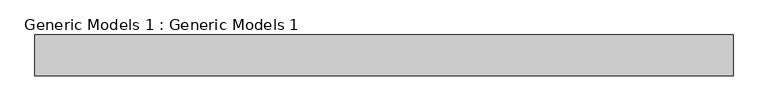
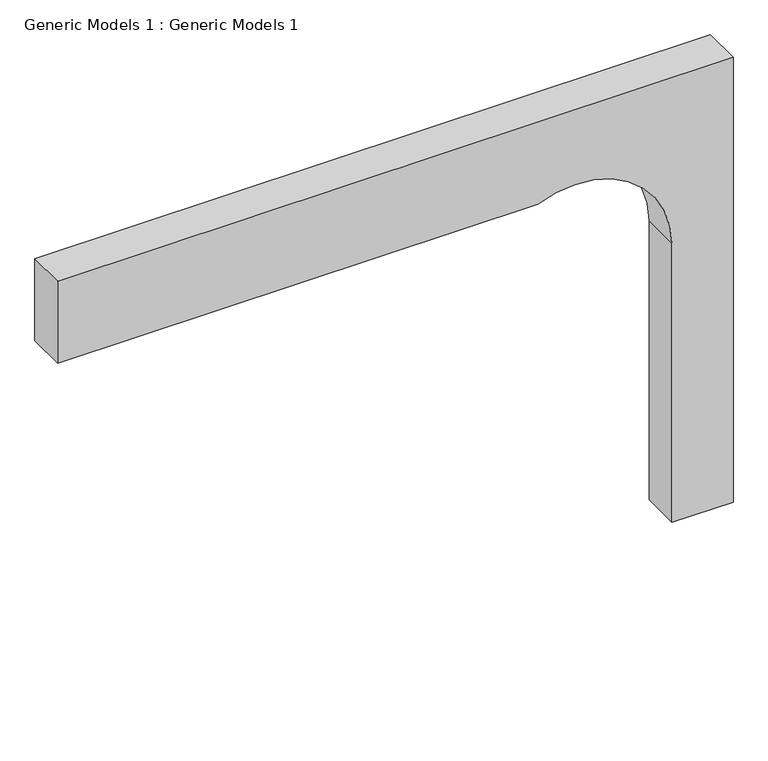
"""IFC4 building model written with IfcOpenShell, lengths in millimetres: proxy geometry, Generic Models 1 : Generic Models 1."""

from ifc_helpers import new_model, si_unit, point, frame, frame_2d, origin, place, context, project, spatial, polyline, circle_curve, trimmed, segment, composite_curve, outline, extrude, source, transform, mapped, element, save


def generic_models_1_generic_models_1_1816b3d2(model_context):
    return source(origin(), model_context, "Body", "SweptSolid", [
        extrude(outline(composite_curve([segment(polyline([(3640.8722399, -15136.2356484), (3640.8722399, -20368.6358231), (2967.4951536, -20368.6358231), (2967.4951536, -16649.4346835)]), True, "CONTINUOUS"), segment(trimmed(circle_curve(frame_2d((2286.0, -16354.0482046)), 742.7575758), [point((2967.4951536, -16649.4346835))], [point((2286.0, -15611.2906288))], True, "CARTESIAN"), True, "CONTINUOUS"), segment(polyline([(2286.0, -15611.2906288), (0.0, -15611.2906288), (0.0, -15136.2356484), (3640.8722399, -15136.2356484)]), True, "CONTINUOUS")], self_intersect=False)), frame((0.0, -4864.6088252, 0.0), z_axis=(0.0, 1.0, 0.0), x_axis=(0.0, 0.0, 1.0)), (0.0, 0.0, 1.0), 304.8),
    ])


if __name__ == "__main__":
    model = new_model("IFC4")
    model_context = context("Model", 3, world=origin())
    ifc_project = project(units=[si_unit("LENGTHUNIT", "METRE", prefix="MILLI")], contexts=[model_context])
    site = spatial("IfcSite", under=ifc_project)
    building = spatial("IfcBuilding", under=site)
    placement = place(None, origin())
    generic_models_1_generic_models_1_shape = generic_models_1_generic_models_1_1816b3d2(model_context)
    element("IfcBuildingElementProxy", 1, Name="Generic Models 1 : Generic Models 1", ObjectType="Generic Models 1 : Generic Models 1", at=placement, inside=building, context=model_context, shape_type="MappedRepresentation", body=[
        mapped(generic_models_1_generic_models_1_shape, transform((0.0, 0.0, 0.0), x_axis=(1.0, 0.0, 0.0), y_axis=(0.0, 1.0, 0.0), z_axis=(0.0, 0.0, 1.0))),
    ])
    save(model, "model.ifc")
